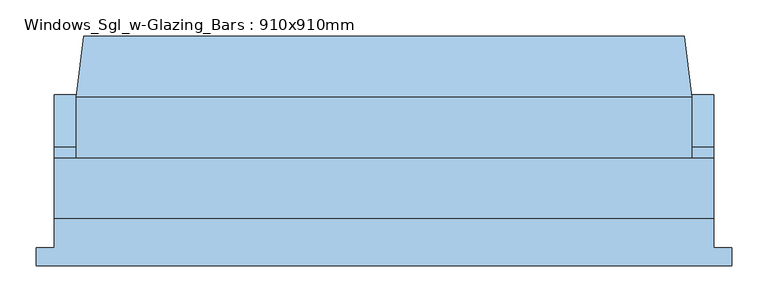
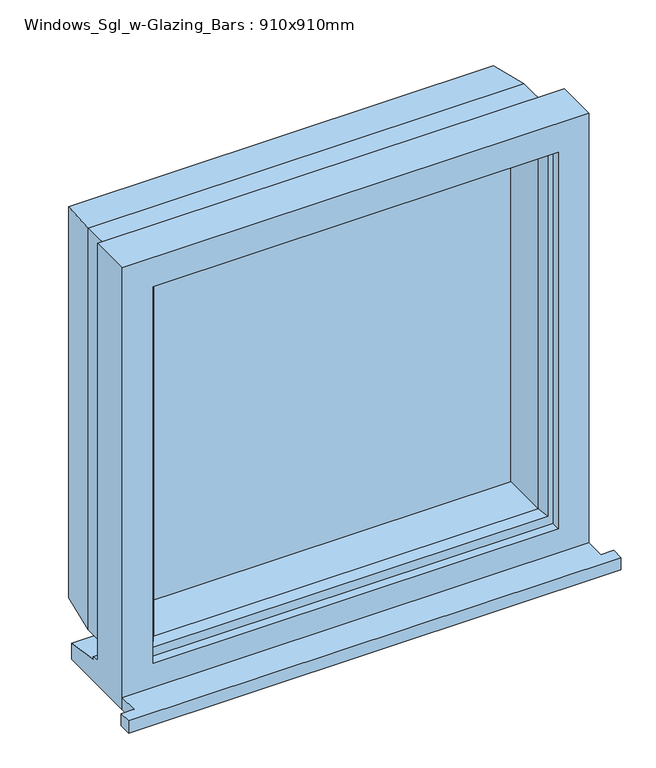
"""IFC4 building model written with IfcOpenShell, lengths in millimetres: window geometry, Windows_Sgl_w-Glazing_Bars : 910x910mm."""

from ifc_helpers import new_model, si_unit, frame, origin, place, context, project, spatial, polyline, outline, extrude, faceted_brep, source, transform, mapped, element, save


def windows_sgl_w_glazing_bars_910x910mm_256712d0(model_context):
    return source(origin(), model_context, "Body", "SolidModel", [
        extrude(outline(polyline([(-480.0, -118.1434322), (-480.0, -93.1434322), (-455.0, -93.1434322), (-455.0, -52.9434322), (455.0, -52.9434322), (455.0, -93.1434322), (480.0, -93.1434322), (480.0, -118.1434322), (-480.0, -118.1434322)])), frame((0.0, 0.0, 1200.0), z_axis=(0.0, 0.0, 1.0), x_axis=(1.0, 0.0, 0.0)), (0.0, 0.0, 1.0), 25.0),
        faceted_brep([(-425.0, 30.0565678, 2080.0), (-425.0, 114.2300705, 2080.0), (-425.0, 114.2300705, 1253.0), (-425.0, 30.0565678, 1253.0), (-415.0, -34.9434322, 2070.0), (-415.0, 30.0565678, 2070.0), (-415.0, 30.0565678, 1263.0), (-415.0, -34.9434322, 1263.0), (-375.0, -20.4505323, 2030.0), (-385.1480377, -34.9434322, 2040.1480377), (-385.1480377, -34.9434322, 1292.8519623), (-375.0, -20.4505323, 1303.0), (-375.0, 72.4565678, 2030.0), (-375.0, 72.4565678, 1303.0), (-385.0, 96.4565678, 2040.0), (-385.0, 72.4565678, 2040.0), (-385.0, 72.4565678, 1293.0), (-385.0, 96.4565678, 1293.0), (-375.0, 114.2300705, 2030.0), (-375.0, 96.4565678, 2030.0), (-375.0, 96.4565678, 1303.0), (-375.0, 114.2300705, 1303.0), (-392.4457548, 198.4035732, 2047.4457548), (-392.4457548, 198.4035732, 1285.5542452), (-414.2153903, 198.4035732, 2069.2153903), (-414.2153903, 198.4035732, 1263.7846097), (425.0, 114.2300705, 1253.0), (425.0, 30.0565678, 1253.0), (415.0, 30.0565678, 1263.0), (415.0, -34.9434322, 1263.0), (385.1480377, -34.9434322, 1292.8519623), (375.0, -20.4505323, 1303.0), (375.0, 72.4565678, 1303.0), (385.0, 72.4565678, 1293.0), (385.0, 96.4565678, 1293.0), (375.0, 96.4565678, 1303.0), (375.0, 114.2300705, 1303.0), (392.4457548, 198.4035732, 1285.5542452), (414.2153903, 198.4035732, 1263.7846097), (425.0, 114.2300705, 2080.0), (425.0, 30.0565678, 2080.0), (415.0, 30.0565678, 2070.0), (415.0, -34.9434322, 2070.0), (385.1480377, -34.9434322, 2040.1480377), (375.0, -20.4505323, 2030.0), (375.0, 72.4565678, 2030.0), (385.0, 72.4565678, 2040.0), (385.0, 96.4565678, 2040.0), (375.0, 96.4565678, 2030.0), (375.0, 114.2300705, 2030.0), (392.4457548, 198.4035732, 2047.4457548), (414.2153903, 198.4035732, 2069.2153903)], [[[0, 1, 2, 3]], [[4, 5, 6, 7]], [[8, 9, 10, 11]], [[12, 8, 11, 13]], [[14, 15, 16, 17]], [[18, 19, 20, 21]], [[22, 18, 21, 23]], [[1, 24, 25, 2]], [[3, 2, 26, 27]], [[7, 6, 28, 29]], [[11, 10, 30, 31]], [[13, 11, 31, 32]], [[17, 16, 33, 34]], [[21, 20, 35, 36]], [[23, 21, 36, 37]], [[2, 25, 38, 26]], [[27, 26, 39, 40]], [[29, 28, 41, 42]], [[31, 30, 43, 44]], [[32, 31, 44, 45]], [[34, 33, 46, 47]], [[36, 35, 48, 49]], [[37, 36, 49, 50]], [[26, 38, 51, 39]], [[40, 39, 1, 0]], [[3, 27, 40, 0], [5, 41, 28, 6]], [[42, 41, 5, 4]], [[7, 29, 42, 4], [9, 43, 30, 10]], [[44, 43, 9, 8]], [[45, 44, 8, 12]], [[15, 46, 33, 16], [13, 32, 45, 12]], [[47, 46, 15, 14]], [[17, 34, 47, 14], [19, 48, 35, 20]], [[49, 48, 19, 18]], [[50, 49, 18, 22]], [[24, 51, 38, 25], [23, 37, 50, 22]], [[39, 51, 24, 1]]]),
        extrude(outline(polyline([(1656.5, 10.0), (1656.5, 385.1480377), (1676.5, 385.1480377), (1676.5, 10.0), (2040.1480377, 10.0), (2040.1480377, -10.0), (1676.5, -10.0), (1676.5, -385.1480377), (1656.5, -385.1480377), (1656.5, -10.0), (1292.8519623, -10.0), (1292.8519623, 10.0), (1656.5, 10.0)])), frame((0.0, 80.4565678, 0.0), z_axis=(0.0, 1.0, 0.0), x_axis=(0.0, 0.0, 1.0)), (0.0, 0.0, 1.0), 8.0),
        faceted_brep([(-455.0, -52.9434322, 1200.0), (455.0, -52.9434322, 1200.0), (455.0, -52.9434322, 2110.0), (-455.0, -52.9434322, 2110.0), (-395.0, -52.9434322, 2050.0), (395.0, -52.9434322, 2050.0), (395.0, -52.9434322, 1275.0), (-395.0, -52.9434322, 1275.0), (-455.0, 30.0565678, 2110.0), (-455.0, 30.0565678, 1251.0), (-455.0, 45.0565678, 1249.68767), (-455.0, 45.0565678, 1244.7449676), (-455.0, 117.5565678, 1233.8088847), (-455.0, 117.5565678, 1200.0), (455.0, 30.0565678, 2110.0), (455.0, 30.0565678, 1251.0), (-415.0, 30.0565678, 2070.0), (-415.0, 30.0565678, 1263.0), (415.0, 30.0565678, 1263.0), (415.0, 30.0565678, 2070.0), (-415.0, -34.9434322, 2070.0), (-415.0, -34.9434322, 1263.0), (415.0, -34.9434322, 2070.0), (415.0, -34.9434322, 1263.0), (-395.0, -34.9434322, 2050.0), (-395.0, -34.9434322, 1275.0), (395.0, -34.9434322, 1275.0), (395.0, -34.9434322, 2050.0), (455.0, 117.5565678, 1200.0), (455.0, 117.5565678, 1233.8088847), (455.0, 45.0565678, 1244.7449676), (455.0, 45.0565678, 1249.68767)], [[[0, 1, 2, 3], [4, 5, 6, 7]], [[0, 3, 8, 9, 10, 11, 12, 13]], [[9, 8, 14, 15], [16, 17, 18, 19]], [[17, 16, 20, 21]], [[20, 22, 23, 21], [24, 25, 26, 27]], [[24, 4, 7, 25]], [[3, 2, 14, 8]], [[16, 19, 22, 20]], [[5, 4, 24, 27]], [[15, 14, 2, 1, 28, 29, 30, 31]], [[19, 18, 23, 22]], [[5, 27, 26, 6]], [[28, 1, 0, 13]], [[29, 28, 13, 12]], [[30, 29, 12, 11]], [[31, 30, 11, 10]], [[15, 31, 10, 9]], [[21, 23, 18, 17]], [[7, 6, 26, 25]]]),
        extrude(outline(polyline([(385.1480377, 72.4565678), (-385.0, 72.4565678), (-385.0, 96.4565678), (385.1480377, 96.4565678), (385.1480377, 72.4565678)])), frame((0.0, 0.0, 1293.0), z_axis=(0.0, 0.0, 1.0), x_axis=(1.0, 0.0, 0.0)), (0.0, 0.0, 1.0), 747.1480377),
    ])


if __name__ == "__main__":
    model = new_model("IFC4")
    model_context = context("Model", 3, world=origin())
    ifc_project = project(units=[si_unit("LENGTHUNIT", "METRE", prefix="MILLI")], contexts=[model_context])
    site = spatial("IfcSite", under=ifc_project)
    building = spatial("IfcBuilding", under=site)
    placement = place(None, origin())
    windows_sgl_w_glazing_bars_910x910mm_shape = windows_sgl_w_glazing_bars_910x910mm_256712d0(model_context)
    element("IfcWindow", 1, ObjectType="Windows_Sgl_w-Glazing_Bars : 910x910mm", at=placement, inside=building, context=model_context, shape_type="MappedRepresentation", body=[
        mapped(windows_sgl_w_glazing_bars_910x910mm_shape, transform((0.0, 0.0, 0.0), x_axis=(1.0, 0.0, 0.0), y_axis=(0.0, 1.0, 0.0), z_axis=(0.0, 0.0, 1.0))),
    ])
    save(model, "model.ifc")

# Revit data of these elements
# Type "Windows_Sgl_w-Glazing_Bars : 910x910mm"
#   Type Mark = "24"
#   Operation = "SinglePanel"
#   Construction Type Id = "SGL"
#   Manufacturer = "Revit"
#   Keynote = "L10"
#   Analytic Construction = "Large single-glazed windows"
#   Wrap Layers (Ext) from Ext = 0' - 4.03543"
#   Wrap Layers (Int) from Ext = 0' - 6.98819"
#   Window Board Projection = 0' - 0.98425"
#   Window Board Extension = 0' - 0.98425"
#   Visual Light Transmittance = 0.9
#   Solar Heat Gain Coefficient = 0.86
#   Rough Width = 2' - 11.82677"
#   Rough Height = 2' - 11.82677"
#   Height = 2' - 11.82677"
#   Width = 2' - 11.82677"
#   Heat Transfer Coefficient (U) = 0.979472 BTU/(h·ft²·°F)
#   Glazing Thickness = 0' - 0.94488"
#   Glazing Bar Thickness = 0' - 0.7874"
#   FrameOffset - External = 0' - 3.14961"
#   Frame Depth = 0' - 2.55906"
#   Default Head Height = 6' - 11.07087"
#   Cill Depth = 0' - 3.44488"
#   Cavity Closer Width = 0' - 1.9685"
#   Cavity Closer Offset from Ext = 0' - 4.03543"
#   Cavity Closer Depth = 0' - 3.34646"
#   Vis - Glazing Bars = yes
#   Vis - Cavity Closers = yes
#   Define Thermal Properties by = 1
#   Material Trim = Window Frame
#   Material Glazing Bars = Window Frame
#   Material Glass = Glass
#   Material Frame = Window Frame
#   Wall Closure = (empty or 0)
# Element 1 (IfcWindow, "Windows_Sgl_w-Glazing_Bars : 910x910mm")
#   Materials on its faces: "Window Frame", "Glass"
# Materials
#   "Window Frame": colour RGB 249 249 249, transparency 0
#   "Glass": class "Glass", colour RGB 0 128 192, transparency 0.75, Description = "Soda Lime Glass", Cost = 0
